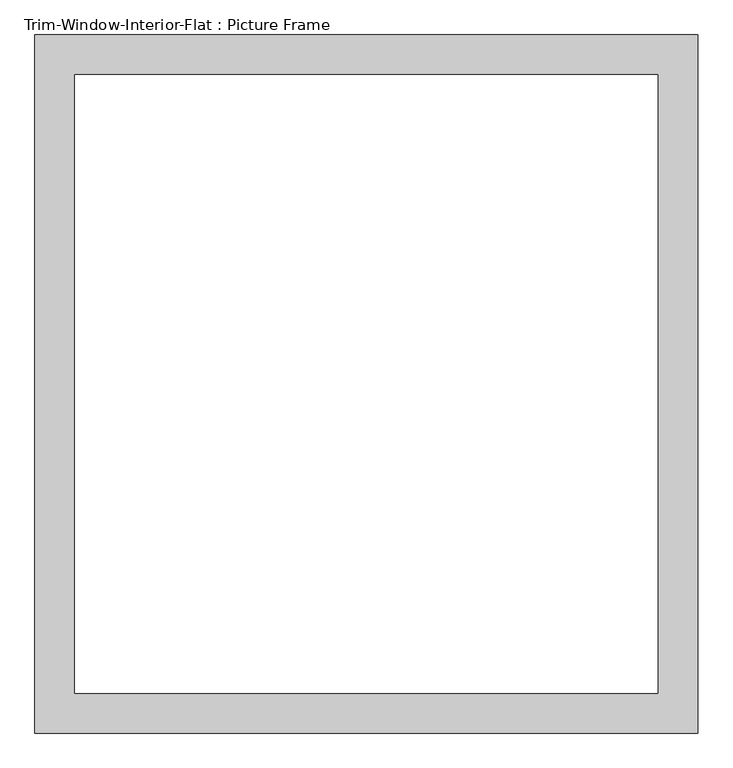
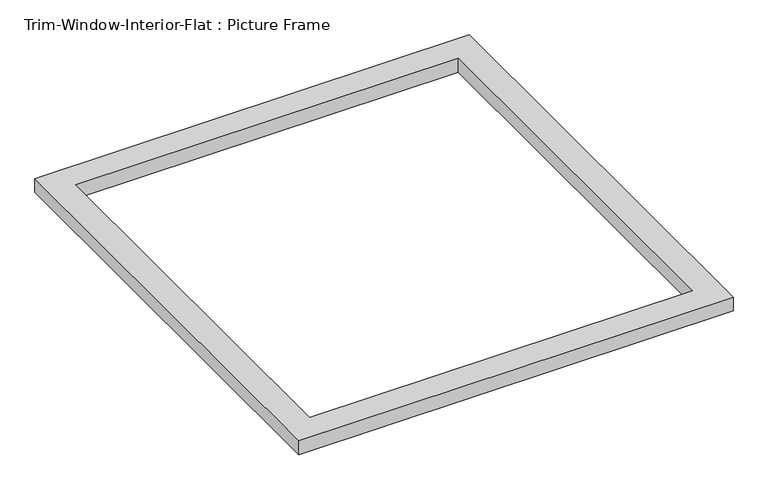
"""IFC4 building model written with IfcOpenShell, lengths in millimetres: proxy geometry, Trim-Window-Interior-Flat : Picture Frame."""

from ifc_helpers import new_model, si_unit, origin, origin_with_axes, place, context, project, spatial, polyline, outline, extrude, source, transform, mapped, element, save


def trim_window_interior_flat_picture_frame_51c85655(model_context):
    return source(origin(), model_context, "Body", "SweptSolid", [
        extrude(outline(polyline([(476.25, 44.45), (476.25, -958.85), (-476.25, -958.85), (-476.25, 44.45), (476.25, 44.45)]), holes=[polyline([(419.1, -12.7), (-419.1, -12.7), (-419.1, -901.7), (419.1, -901.7), (419.1, -12.7)])]), origin_with_axes(), (0.0, 0.0, 1.0), 31.75),
    ])


if __name__ == "__main__":
    model = new_model("IFC4")
    model_context = context("Model", 3, world=origin())
    ifc_project = project(units=[si_unit("LENGTHUNIT", "METRE", prefix="MILLI")], contexts=[model_context])
    site = spatial("IfcSite", under=ifc_project)
    building = spatial("IfcBuilding", under=site)
    placement = place(None, origin())
    trim_window_interior_flat_picture_frame_shape = trim_window_interior_flat_picture_frame_51c85655(model_context)
    element("IfcBuildingElementProxy", 1, Name="Trim-Window-Interior-Flat : Picture Frame", ObjectType="Trim-Window-Interior-Flat : Picture Frame", at=placement, inside=building, context=model_context, shape_type="MappedRepresentation", body=[
        mapped(trim_window_interior_flat_picture_frame_shape, transform((0.0, 0.0, 0.0), x_axis=(1.0, 0.0, 0.0), y_axis=(0.0, 1.0, 0.0), z_axis=(0.0, 0.0, 1.0))),
    ])
    save(model, "model.ifc")

# Revit data of these elements
# Type "Trim-Window-Interior-Flat : Picture Frame"
#   Trim Thickness_Picture Frame = 1.25"
#   Trim Width = 2.25"
#   Trim Thickness_with Sill = 0.75"
#   Sill Thickness = 1.25"
#   Opening Width [instance default] = 24"
#   Opening Height [instance default] = 36"
#   Default Elevation = 48"
#   Sill = no
#   Picture Frame = yes
#   Trim Material [instance default] = none
# Element 1 (IfcBuildingElementProxy, "Trim-Window-Interior-Flat : Picture Frame")
#   Opening Width = 34"
#   Trim Material = Wood - Stained
#   Materials on its faces: "Wood - Stained"
# Materials
#   "Wood - Stained": class "Wood", colour RGB 224 178 126, transparency 0, Cost = 0
